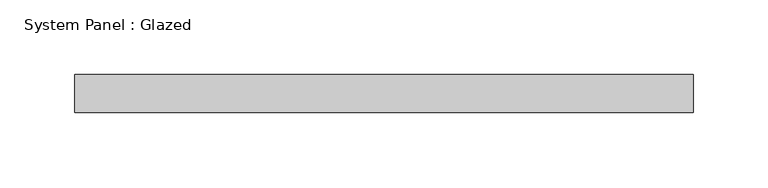
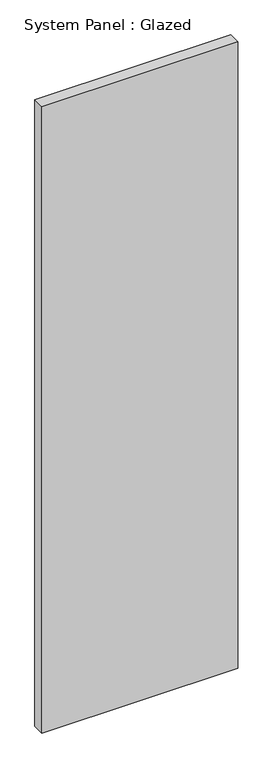
"""IFC4 building model written with IfcOpenShell, lengths in millimetres: plate geometry, System Panel : Glazed."""

from ifc_helpers import new_model, si_unit, origin, origin_with_axes, place, context, project, spatial, polyline, outline, extrude, source, transform, mapped, element, save


def system_panel_glazed_6aba1888(model_context):
    return source(origin(), model_context, "Body", "SweptSolid", [
        extrude(outline(polyline([(206.375, 19.05), (-206.375, 19.05), (-206.375, 44.45), (206.375, 44.45), (206.375, 19.05)])), origin_with_axes(), (0.0, 0.0, 1.0), 1395.1457324),
    ])


if __name__ == "__main__":
    model = new_model("IFC4")
    model_context = context("Model", 3, world=origin())
    ifc_project = project(units=[si_unit("LENGTHUNIT", "METRE", prefix="MILLI")], contexts=[model_context])
    site = spatial("IfcSite", under=ifc_project)
    building = spatial("IfcBuilding", under=site)
    placement = place(None, origin())
    system_panel_glazed_shape = system_panel_glazed_6aba1888(model_context)
    element("IfcPlate", 1, ObjectType="System Panel : Glazed", at=placement, inside=building, context=model_context, shape_type="MappedRepresentation", body=[
        mapped(system_panel_glazed_shape, transform((0.0, 0.0, 0.0), x_axis=(1.0, 0.0, 0.0), y_axis=(0.0, 1.0, 0.0), z_axis=(0.0, 0.0, 1.0))),
    ])
    save(model, "model.ifc")

# Revit data of these elements
# Type "System Panel : Glazed"
#   Construction Type Id = "GSP4R"
#   Analytic Construction = "1/8 in Pilkington single glazing"
#   Visual Light Transmittance = 0.9
#   Solar Heat Gain Coefficient = 0.86
#   Heat Transfer Coefficient (U) = 1.18115 BTU/(h·ft²·°F)
#   Define Thermal Properties by = 1
# Element 1 (IfcPlate, "System Panel : Glazed")
#   Materials on its faces: "Glass"
# Materials
#   "Glass": class "Glass", colour RGB 0 128 192, transparency 0.75, Description = "Soda Lime Glass", Cost = 0
